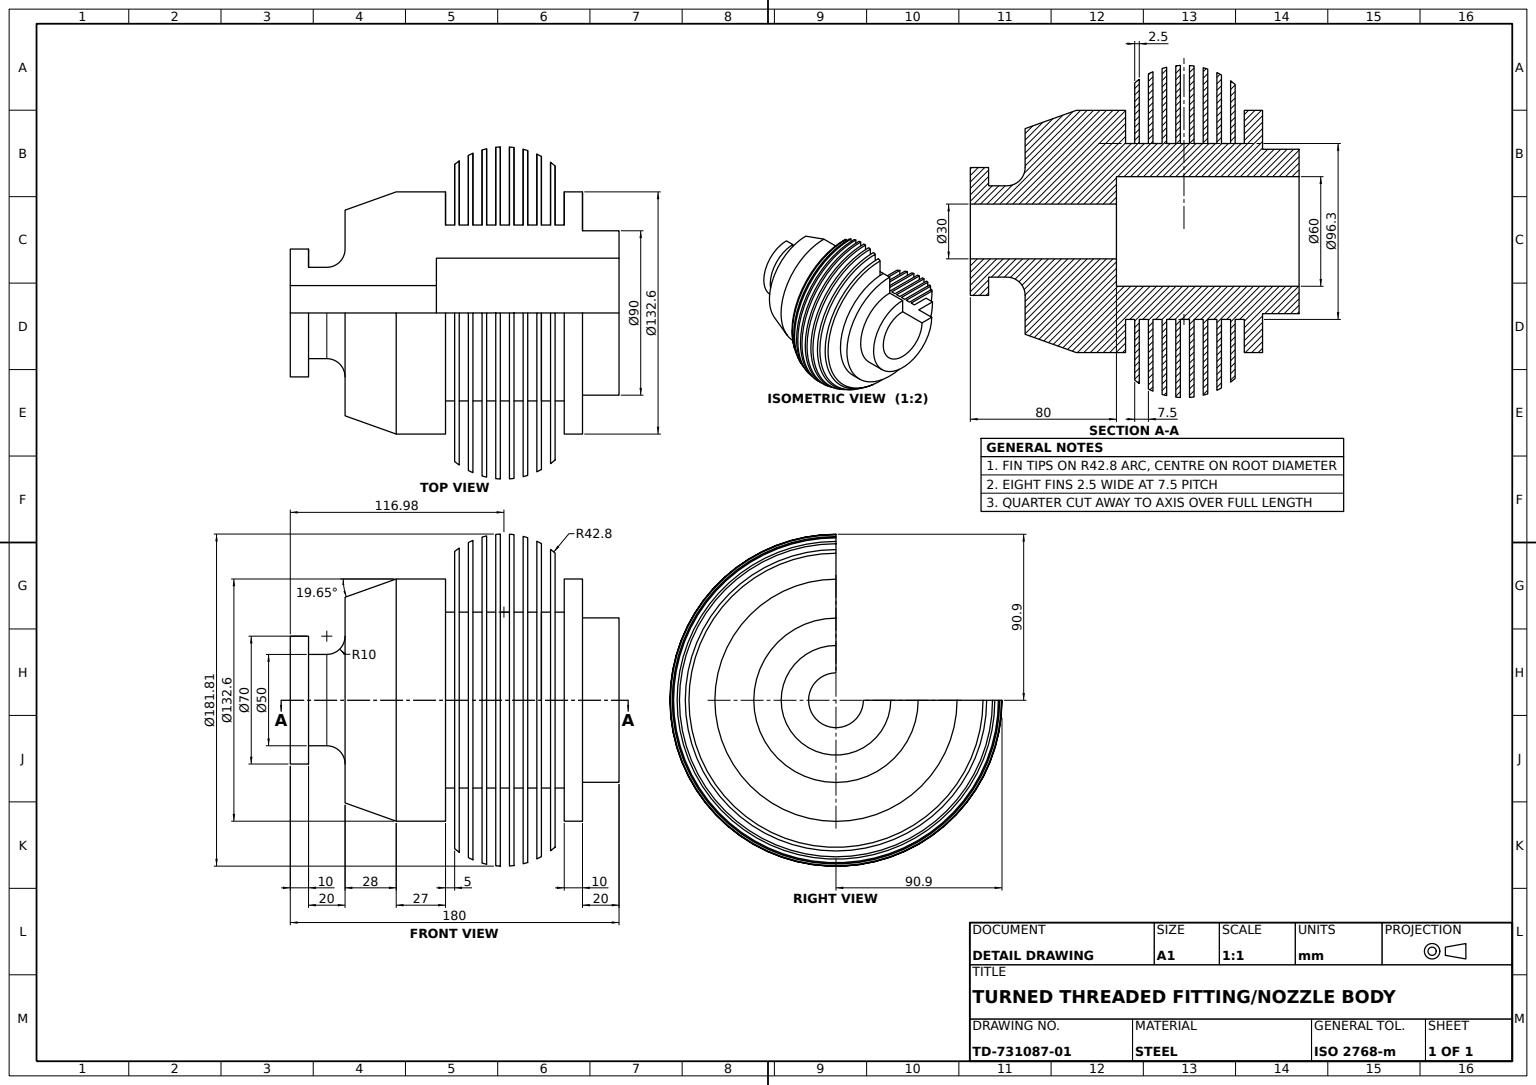
from build123d import *

# Parameters (mm, degrees)
SLOT_CUT_DEPTH      = 81
SLOT_CUT_DEPTH_BACK = 267
SLOT_CUT_SKETCH_W   = 99.104546372
SLOT_CUT_SKETCH_H   = 99.716302831


with BuildPart() as part:
    # Shaft Profile Sketch → Revolved Shaft Body (revolve)
    with BuildSketch(Plane(origin=(0, 0, 0), x_dir=(1, 0, 0), z_dir=(0, 1, 0)), mode=Mode.PRIVATE) as revolved_shaft_body_sk:
        with BuildLine():
            Line((51.156388298, 36.67448577), (51.156388298, 51.67448577))
            Line((51.156388298, 51.67448577), (31.156388298, 51.67448577))
            Line((31.156388298, 51.67448577), (31.156388298, 72.97448577))
            Line((31.156388298, 72.97448577), (21.156388298, 72.97448577))
            Line((21.156388298, 72.97448577), (21.156388298, 54.82448577))
            Line((21.156388298, 54.82448577), (16.156388298, 54.82448577))
            Line((16.156388298, 54.82448577), (16.156388298, 75.255525061))
            Line((16.156388298, 75.255525061), (16.156388298, 87.176546037))
            ThreePointArc((16.156388298, 87.176546037), (14.925180355, 88.203215925), (13.656388298, 89.183058142))
            Line((13.656388298, 89.183058142), (13.656388298, 75.255525061))
            Line((13.656388298, 75.255525061), (13.656388298, 54.82448577))
            Line((13.656388298, 54.82448577), (8.656388298, 54.82448577))
            Line((8.656388298, 54.82448577), (8.656388298, 75.255525061))
            Line((8.656388298, 75.255525061), (8.656388298, 92.384076813))
            ThreePointArc((8.656388298, 92.384076813), (7.416708158, 93.035287487), (6.156388298, 93.645595636))
            Line((6.156388298, 93.645595636), (6.156388298, 75.255525061))
            Line((6.156388298, 75.255525061), (6.156388298, 54.82448577))
            Line((6.156388298, 54.82448577), (1.156388298, 54.82448577))
            Line((1.156388298, 54.82448577), (1.156388298, 75.255525061))
            Line((1.156388298, 75.255525061), (1.156388298, 95.595676029))
            ThreePointArc((1.156388298, 95.595676029), (-0.088176532, 95.972417859), (-1.343611702, 96.311178179))
            Line((-1.343611702, 96.311178179), (-1.343611702, 75.255525061))
            Line((-1.343611702, 75.255525061), (-1.343611702, 54.82448577))
            Line((-1.343611702, 54.82448577), (-6.343611702, 54.82448577))
            Line((-6.343611702, 54.82448577), (-6.343611702, 75.255525061))
            Line((-6.343611702, 75.255525061), (-6.343611702, 97.266882391))
            ThreePointArc((-6.343611702, 97.266882391), (-7.591770603, 97.410653082), (-8.843611702, 97.517725549))
            Line((-8.843611702, 97.517725549), (-8.843611702, 92.720576379))
            Line((-8.843611702, 92.720576379), (-8.843611702, 75.255525061))
            Line((-8.843611702, 75.255525061), (-8.843611702, 54.82448577))
            Line((-8.843611702, 54.82448577), (-13.843611702, 54.82448577))
            Line((-13.843611702, 54.82448577), (-13.843611702, 75.255525061))
            Line((-13.843611702, 75.255525061), (-13.843611702, 97.578714879))
            ThreePointArc((-13.843611702, 97.578714879), (-15.09499754, 97.502413337), (-16.343611702, 97.389492508))
            Line((-16.343611702, 97.389492508), (-16.343611702, 75.255525061))
            Line((-16.343611702, 75.255525061), (-16.343611702, 54.82448577))
            Line((-16.343611702, 54.82448577), (-21.343611702, 54.82448577))
            Line((-21.343611702, 54.82448577), (-21.343611702, 75.255525061))
            Line((-21.343611702, 75.255525061), (-21.343611702, 96.561653648))
            ThreePointArc((-21.343611702, 96.561653648), (-22.598497826, 96.256679286), (-23.843611702, 95.913984117))
            Line((-23.843611702, 95.913984117), (-23.843611702, 75.255525061))
            Line((-23.843611702, 75.255525061), (-23.843611702, 54.82448577))
            Line((-23.843611702, 54.82448577), (-28.843611702, 54.82448577))
            Line((-28.843611702, 54.82448577), (-28.843611702, 75.255525061))
            Line((-28.843611702, 75.255525061), (-28.843611702, 94.112629762))
            ThreePointArc((-28.843611702, 94.112629762), (-30.103118387, 93.544014716), (-31.343611702, 92.935034838))
            Line((-31.343611702, 92.935034838), (-31.343611702, 75.255525061))
            Line((-31.343611702, 75.255525061), (-31.343611702, 54.82448577))
            Line((-31.343611702, 54.82448577), (-36.343611702, 54.82448577))
            Line((-36.343611702, 54.82448577), (-36.343611702, 75.255525061))
            Line((-36.343611702, 75.255525061), (-36.343611702, 89.933250119))
            ThreePointArc((-36.343611702, 89.933250119), (-37.610824017, 89.014830566), (-38.843611702, 88.050695696))
            Line((-38.843611702, 88.050695696), (-38.843611702, 75.255525061))
            Line((-38.843611702, 75.255525061), (-38.843611702, 54.82448577))
            Line((-38.843611702, 54.82448577), (-43.843611702, 54.82448577))
            Line((-43.843611702, 54.82448577), (-43.843611702, 72.97448577))
            Line((-43.843611702, 72.97448577), (-70.843611702, 72.97448577))
            Line((-70.843611702, 72.97448577), (-98.843611702, 62.97448577))
            Line((-98.843611702, 62.97448577), (-98.843611702, 41.67448577))
            ThreePointArc((-98.843611702, 41.67448577), (-101.772543891, 34.603417958), (-108.843611702, 31.67448577))
            Line((-108.843611702, 31.67448577), (-118.843611702, 31.67448577))
            Line((-118.843611702, 31.67448577), (-118.843611702, 41.67448577))
            Line((-118.843611702, 41.67448577), (-128.843611702, 41.67448577))
            Line((-128.843611702, 41.67448577), (-128.843611702, 21.67448577))
            Line((-128.843611702, 21.67448577), (-48.843611702, 21.67448577))
            Line((-48.843611702, 21.67448577), (-48.843611702, 36.67448577))
            Line((-48.843611702, 36.67448577), (51.156388298, 36.67448577))
        make_face()
    revolve(revolved_shaft_body_sk.sketch.rotate(Axis((-149.605779726, 0, -6.67448577), (1, 0, 0)), 180), axis=Axis((-149.605779726, 0, -6.67448577), (1, 0, 0)))

    # Slot Cut Sketch → Slot Cut (cut, two sides: drawn at the far end of the back side and taken through both)
    with BuildSketch(Plane(origin=(51.156388298, 0, 0), x_dir=(0, 0, -1), z_dir=(1, 0, 0)).offset(-SLOT_CUT_DEPTH_BACK)):
        with Locations((56.226758956, 49.858151416)):
            Rectangle(SLOT_CUT_SKETCH_W, SLOT_CUT_SKETCH_H)
    extrude(amount=SLOT_CUT_DEPTH + SLOT_CUT_DEPTH_BACK, mode=Mode.SUBTRACT)


solid = part.part
